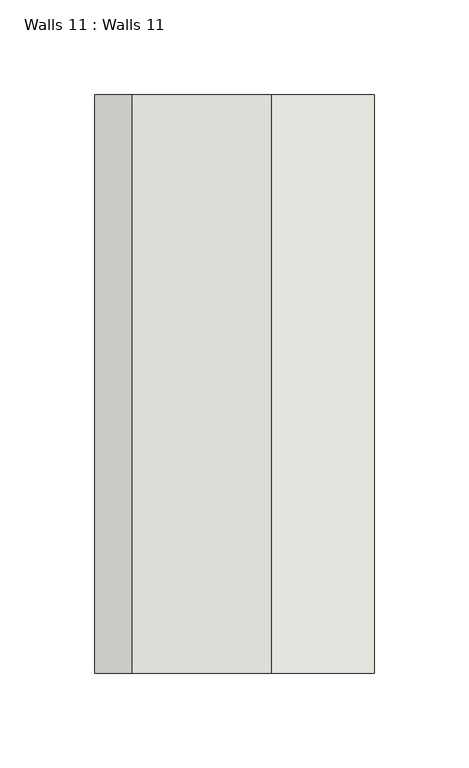
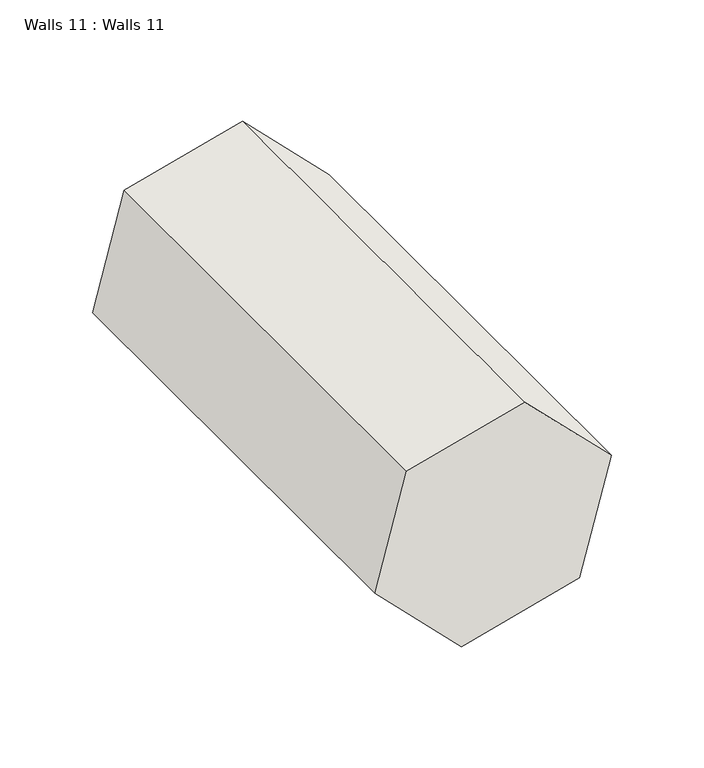
"""IFC4 building model written with IfcOpenShell, lengths in millimetres: wall geometry, Walls 11 : Walls 11."""

from ifc_helpers import new_model, si_unit, frame, origin, place, context, project, spatial, polyline, outline, extrude, source, transform, mapped, element, save


def walls_11_walls_11_7ea3dec3(model_context):
    return source(origin(), model_context, "Body", "SweptSolid", [
        extrude(outline(polyline([(667.8155515, -8814.7125877), (721.6970882, -8868.5941244), (701.975077, -8942.1976723), (628.371529, -8961.9196836), (574.4899923, -8908.0381469), (594.2120035, -8834.4345989), (667.8155515, -8814.7125877)])), frame((0.0, 3351.3956099, 0.0), z_axis=(0.0, 1.0, 0.0), x_axis=(0.0, 0.0, 1.0)), (0.0, 0.0, 1.0), 304.8),
    ])


if __name__ == "__main__":
    model = new_model("IFC4")
    model_context = context("Model", 3, world=origin())
    ifc_project = project(units=[si_unit("LENGTHUNIT", "METRE", prefix="MILLI")], contexts=[model_context])
    site = spatial("IfcSite", under=ifc_project)
    building = spatial("IfcBuilding", under=site)
    placement = place(None, origin())
    walls_11_walls_11_shape = walls_11_walls_11_7ea3dec3(model_context)
    element("IfcWall", 1, ObjectType="Walls 11 : Walls 11", at=placement, inside=building, context=model_context, shape_type="MappedRepresentation", body=[
        mapped(walls_11_walls_11_shape, transform((0.0, 0.0, 0.0), x_axis=(1.0, 0.0, 0.0), y_axis=(0.0, 1.0, 0.0), z_axis=(0.0, 0.0, 1.0))),
    ])
    save(model, "model.ifc")

# Revit data of these elements
# Element 1 (IfcWall, "Walls 11 : Walls 11")
#   Materials on its faces: "Default Wall"
# Materials
#   "Default Wall": colour RGB 80 80 80, transparency 0
